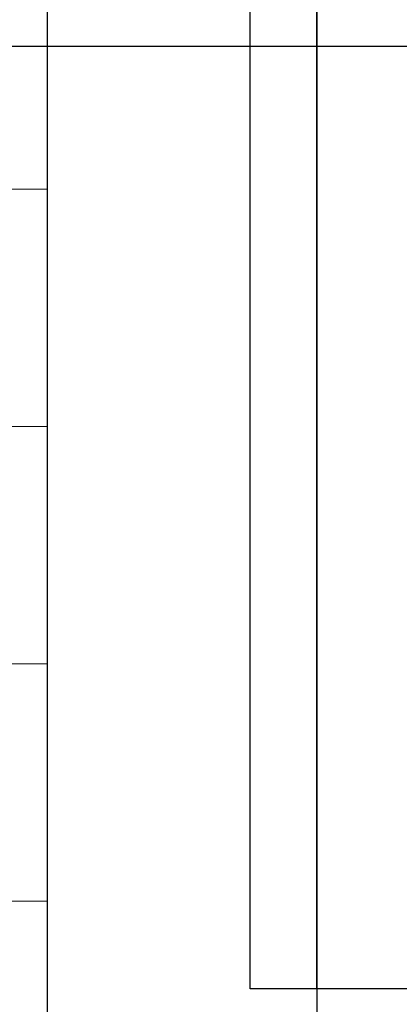
# Model space of a CAD drawing. Units: inches. Extents: x 37 to 824, y -700 to 234.
# Tile 12 of 77: x 298 to 315, y -581 to -536. Entities that reach past the tile are written whole.
import ezdxf

# ---------------------------------------------------------------- set-up
doc = ezdxf.new("R2010")
doc.units = ezdxf.units.IN
doc.header["$MEASUREMENT"] = 0
for name, color, linetype, lineweight in [('A-ANNO-DIMS', 2, 'Continuous', 18), ('A-DOOR', 4, 'Continuous', 25), ('A-ELEV', 3, 'Continuous', 25), ('A-ELEV-PATT', 8, 'Continuous', 13)]:
    doc.layers.add(name, color=color, linetype=linetype, lineweight=lineweight)
doc.styles.get("Standard").update_dxf_attribs({"font": 'arial.ttf'})
doc.dimstyles.get("Standard").update_dxf_attribs({"dimtxt": 0.18, "dimasz": 0.18, "dimexe": 0.18, "dimexo": 0.0625, "dimgap": 0.09, "dimtad": 0, "dimtih": 1, "dimtoh": 1, "dimdec": 1, "dimzin": 0, "dimdsep": 46, "dimlunit": 4, "dimtxsty": 'Standard', "dimcen": 0.09, "dimadec": 0, "dimazin": 0, "dimtfac": 1, "dimtdec": 1, "dimtofl": 0, "dimtmove": 0, "dimatfit": 3, "dimfxl": 1, "dimtolj": 1, "dimtzin": 0, "dimarcsym": 0})

# ---------------------------------------------------------------- blocks, each defined once
blk = doc.blocks.new('*U9')
blk.add_lwpolyline([(3.124, 0.013), (0.124, 0.013), (0.124, 84.013), (40.124, 84.013), (40.124, 0.013), (37.124, 0.013)])
blk.add_lwpolyline([(37.124, 80.99), (37.124, 0.013), (3.124, 0.013), (3.124, 80.99)], close=True)
blk = doc.blocks.new('*D28')
at = {"layer": 'A-ANNO-DIMS', "color": 0, "lineweight": -2, "ltscale": 0.5, "transparency": 16777216}
for p, q in [((255.14, -537.627), (449.868, -537.627)), ((449.688, -543.627), (449.688, -558.537)), ((449.688, -579.627), (449.688, -564.717)), ((294.64, -585.627), (449.868, -585.627))]:
    blk.add_line(p, q, dxfattribs=at)
at = {"layer": 'A-ANNO-DIMS', "color": 0, "ltscale": 0.5, "transparency": 16777216}
for points in [[(448.688, -543.627), (450.688, -543.627), (449.688, -537.627)], [(448.688, -579.627), (450.688, -579.627), (449.688, -585.627)]]:
    blk.add_solid(points, dxfattribs=at)
at = {"layer": 'Defpoints', "color": 0, "ltscale": 0.5, "transparency": 16777216}
for p in [(255.077, -537.627), (294.577, -585.627), (449.688, -585.627)]:
    blk.add_point(p, dxfattribs=at)
at = {"layer": 'A-ANNO-DIMS', "color": 0, "ltscale": 0.5, "transparency": 16777216, "insert": (449.688, -561.627), "char_height": 6, "attachment_point": 5}
blk.add_mtext("\\A1;4'", dxfattribs=at)
blk = doc.blocks.new('*D31')
at = {"layer": 'A-ANNO-DIMS', "color": 0, "lineweight": -2, "ltscale": 0.5, "transparency": 16777216}
for p, q in [((255.14, -489.627), (449.772, -489.627)), ((449.592, -495.627), (449.592, -510.537)), ((449.592, -531.627), (449.592, -516.717)), ((255.14, -537.627), (449.772, -537.627))]:
    blk.add_line(p, q, dxfattribs=at)
at = {"layer": 'A-ANNO-DIMS', "color": 0, "ltscale": 0.5, "transparency": 16777216}
for points in [[(448.592, -495.627), (450.592, -495.627), (449.592, -489.627)], [(448.592, -531.627), (450.592, -531.627), (449.592, -537.627)]]:
    blk.add_solid(points, dxfattribs=at)
at = {"layer": 'Defpoints', "color": 0, "ltscale": 0.5, "transparency": 16777216}
for p in [(255.077, -489.627), (449.592, -489.627), (255.077, -537.627)]:
    blk.add_point(p, dxfattribs=at)
at = {"layer": 'A-ANNO-DIMS', "color": 0, "ltscale": 0.5, "transparency": 16777216, "insert": (449.592, -513.627), "char_height": 6, "attachment_point": 5}
blk.add_mtext("\\A1;4'", dxfattribs=at)
blk = doc.blocks.new('*D69')
at = {"layer": 'A-ANNO-DIMS', "color": 0, "lineweight": -2, "ltscale": 0.5, "transparency": 16777216}
for p, q in [((255.077, -537.69), (255.077, -699.594)), ((299.077, -585.69), (299.077, -699.594)), ((255.257, -699.414), (276.748, -699.414)), ((298.897, -699.414), (277.406, -699.414))]:
    blk.add_line(p, q, dxfattribs=at)
at = {"layer": 'A-ANNO-DIMS', "color": 0, "ltscale": 0.5, "transparency": 16777216}
for points in [[(255.257, -699.384), (255.257, -699.444), (255.077, -699.414)], [(298.897, -699.384), (298.897, -699.444), (299.077, -699.414)]]:
    blk.add_solid(points, dxfattribs=at)
at = {"layer": 'Defpoints', "color": 0, "ltscale": 0.5, "transparency": 16777216}
for p in [(255.077, -537.627), (299.077, -585.627), (299.077, -699.414)]:
    blk.add_point(p, dxfattribs=at)
at = {"layer": 'A-ANNO-DIMS', "color": 0, "ltscale": 0.5, "transparency": 16777216, "insert": (277.077, -699.414), "char_height": 0.18, "attachment_point": 5}
blk.add_mtext('\\A1;3\'-8"', dxfattribs=at)
blk = doc.blocks.new('*D102')
at = {"layer": 'A-ANNO-DIMS', "color": 0, "lineweight": -2, "ltscale": 0.5, "transparency": 16777216}
for p, q in [((311.196, -499.092), (311.196, -699.594)), ((345.196, -499.092), (345.196, -699.594)), ((311.376, -699.414), (327.795, -699.414)), ((345.016, -699.414), (328.596, -699.414))]:
    blk.add_line(p, q, dxfattribs=at)
at = {"layer": 'A-ANNO-DIMS', "color": 0, "ltscale": 0.5, "transparency": 16777216}
for points in [[(311.376, -699.384), (311.376, -699.444), (311.196, -699.414)], [(345.016, -699.384), (345.016, -699.444), (345.196, -699.414)]]:
    blk.add_solid(points, dxfattribs=at)
at = {"layer": 'Defpoints', "color": 0, "ltscale": 0.5, "transparency": 16777216}
for p in [(311.196, -499.03), (345.196, -499.03), (345.196, -699.414)]:
    blk.add_point(p, dxfattribs=at)
at = {"layer": 'A-ANNO-DIMS', "color": 0, "ltscale": 0.5, "transparency": 16777216, "insert": (328.196, -699.414), "char_height": 0.18, "attachment_point": 5}
blk.add_mtext('\\A1;2\'-10"', dxfattribs=at)

msp = doc.modelspace()

# ---------------------------------------------------------------- hatches: boundary and pattern name
at = {"layer": 'A-ELEV-PATT', "ltscale": 0.5}
h = msp.add_hatch(dxfattribs=at)
h.set_pattern_fill('AR-BRSTD', color=256, scale=4)
h.paths.add_polyline_path([(299.077, -489.627), (358.132, -489.627), (358.132, -585.627), (428.077, -585.627), (428.077, -465.627), (161.077, -465.627), (161.077, -585.627), (299.077, -585.627)])
h.paths.add_polyline_path([(205.077, -537.627), (205.077, -489.627), (255.077, -489.627), (255.077, -537.627)], flags=16)

# ---------------------------------------------------------------- linework, layer by layer
at = {"layer": 'A-ELEV', "ltscale": 0.5}
msp.add_lwpolyline([(299.077, -489.627), (358.132, -489.627), (358.132, -585.627), (299.077, -585.627)], close=True, dxfattribs=at)

# ---------------------------------------------------------------- block references
at = {"layer": 'A-DOOR'}
msp.add_blockref('*U9', (308.072, -580.019), dxfattribs=at)

# ---------------------------------------------------------------- dimensions: what is measured, and where the dimension line sits
at = {"layer": 'A-ANNO-DIMS', "ltscale": 0.5}
for base, p2, picture, middle in [((449.592, -489.627), (255.077, -489.627), '*D31', (449.592, -513.627)), ((449.688, -585.627), (294.577, -585.627), '*D28', (449.688, -561.627))]:
    dim = msp.add_linear_dim(base=base, p1=(255.077, -537.627), p2=p2, angle=90, dimstyle='Standard', override={"dimtxt": 6, "dimasz": 6, "dimclrd": 0, "dimclre": 0, "dimclrt": 0}, dxfattribs=at)
    dim.commit()
    dim.dimension.update_dxf_attribs({"geometry": picture, "text_midpoint": middle})
for base, p1, p2, picture, middle in [((345.196, -699.414), (311.196, -499.03), (345.196, -499.03), '*D102', (328.196, -699.414)), ((299.077, -699.414), (255.077, -537.627), (299.077, -585.627), '*D69', (277.077, -699.414))]:
    dim = msp.add_linear_dim(base=base, p1=p1, p2=p2, dimstyle='Standard', override={"dimdec": 1, "dimlfac": 1, "dimrnd": 0, "dimzin": 1, "dimdsep": 46, "dimlunit": 4, "dimfrac": 2}, dxfattribs=at)
    dim.commit()
    dim.dimension.update_dxf_attribs({"geometry": picture, "text_midpoint": middle})

doc.saveas('drawing.dxf')
